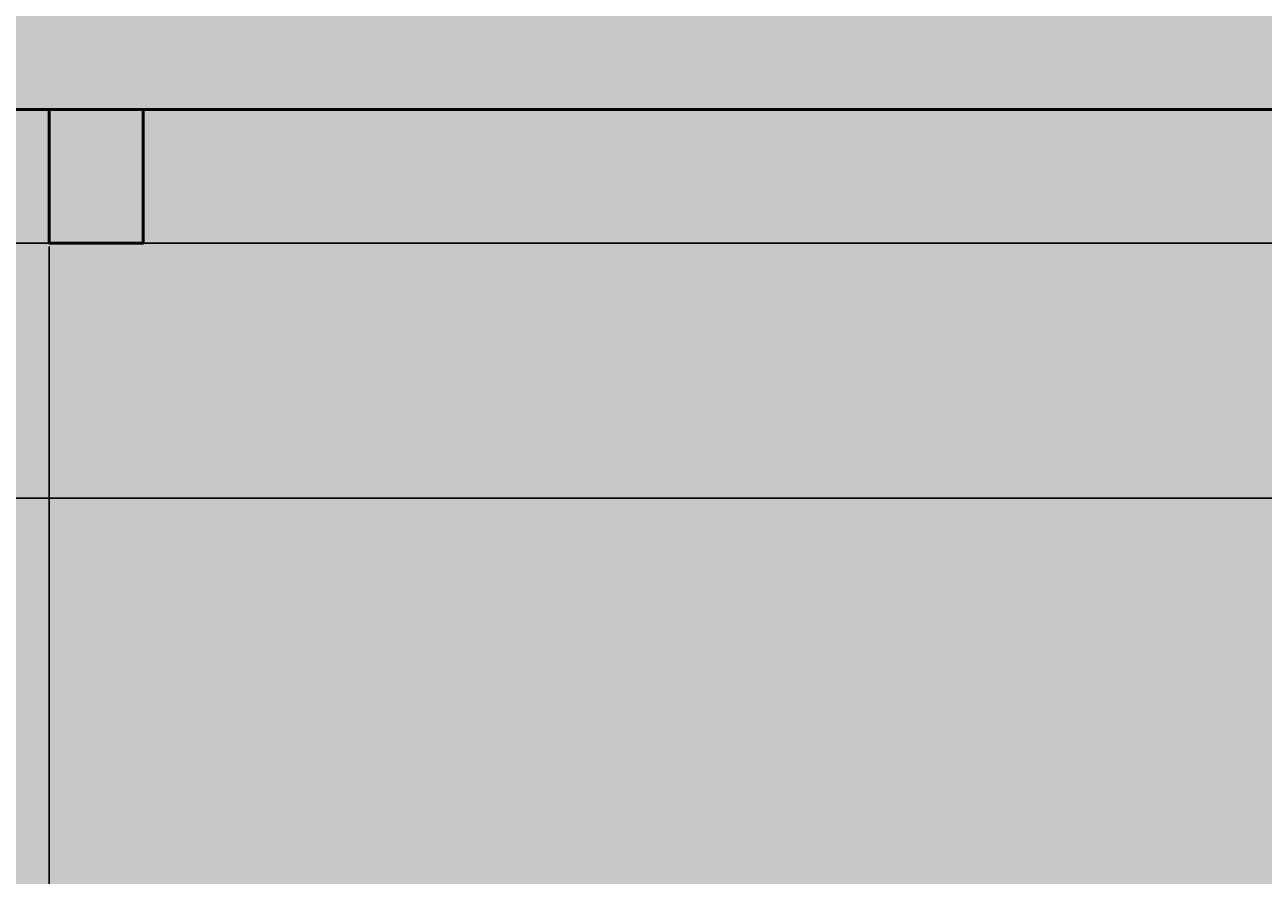
# Model space of a CAD drawing. Units: inches. Extents: x -12 to 334, y -10 to 186.
# Tile 37 of 77: x 129 to 152, y 49 to 65. Entities that reach past the tile are written whole.
import ezdxf

# ---------------------------------------------------------------- set-up
doc = ezdxf.new("R2010")
doc.units = ezdxf.units.IN
doc.header["$MEASUREMENT"] = 0
for name, color, linetype, lineweight in [('M-DIMS', 2, 'Continuous', 18), ('M-EQPM', 7, 'Continuous', 50), ('M-EQPM-PATT', 8, 'Continuous', 18)]:
    doc.layers.add(name, color=color, linetype=linetype, lineweight=lineweight)
doc.styles.get("Standard").update_dxf_attribs({"font": 'arial.ttf'})
doc.dimstyles.get("Standard").update_dxf_attribs({"dimtxt": 0.18, "dimasz": 0.18, "dimexe": 0.18, "dimexo": 0.0625, "dimgap": 0.09, "dimtad": 0, "dimtih": 1, "dimtoh": 1, "dimdec": 4, "dimzin": 0, "dimdsep": 46, "dimtxsty": 'Standard', "dimcen": 0.09, "dimadec": 0, "dimazin": 0, "dimtfac": 1, "dimtdec": 4, "dimtofl": 0, "dimtmove": 0, "dimatfit": 3, "dimfxl": 1, "dimtolj": 1, "dimtzin": 0, "dimarcsym": 0})

# ---------------------------------------------------------------- blocks, each defined once
blk = doc.blocks.new('*D1')
at = {"layer": 'Defpoints', "color": 0, "transparency": 16777216}
for p in [(281.426, 91.899), (3.376, 80.692), (281.426, 14.304)]:
    blk.add_point(p, dxfattribs=at)
at = {"layer": 'M-DIMS', "color": 0, "lineweight": -2, "transparency": 16777216}
for p, q in [((281.426, 91.836), (281.426, 14.124)), ((3.376, 80.629), (3.376, 14.124)), ((3.556, 14.304), (141.935, 14.304)), ((281.246, 14.304), (142.867, 14.304))]:
    blk.add_line(p, q, dxfattribs=at)
at = {"layer": 'M-DIMS', "color": 0, "transparency": 16777216}
for points in [[(3.556, 14.334), (3.556, 14.274), (3.376, 14.304)], [(281.246, 14.334), (281.246, 14.274), (281.426, 14.304)]]:
    blk.add_solid(points, dxfattribs=at)
at = {"layer": 'M-DIMS', "color": 0, "transparency": 16777216, "insert": (142.401, 14.304), "char_height": 0.18, "attachment_point": 5}
blk.add_mtext('\\A1;278.05', dxfattribs=at)
blk = doc.blocks.new('*D17')
at = {"layer": 'Defpoints', "color": 0, "transparency": 16777216}
for p in [(106.177, 102.896), (105.892, 56.321), (295.976, 56.321)]:
    blk.add_point(p, dxfattribs=at)
at = {"layer": 'M-DIMS', "color": 0, "lineweight": -2, "transparency": 16777216}
for p, q in [((106.24, 102.896), (296.156, 102.896)), ((295.976, 102.716), (295.976, 79.79)), ((295.976, 56.501), (295.976, 79.426)), ((105.954, 56.321), (296.156, 56.321))]:
    blk.add_line(p, q, dxfattribs=at)
at = {"layer": 'M-DIMS', "color": 0, "transparency": 16777216}
for points in [[(295.946, 102.716), (296.006, 102.716), (295.976, 102.896)], [(295.946, 56.501), (296.006, 56.501), (295.976, 56.321)]]:
    blk.add_solid(points, dxfattribs=at)
at = {"layer": 'M-DIMS', "color": 0, "transparency": 16777216, "insert": (295.976, 79.608), "char_height": 0.18, "attachment_point": 5}
blk.add_mtext('\\A1;46.575', dxfattribs=at)
blk = doc.blocks.new('*D30')
at = {"layer": 'Defpoints', "color": 0, "transparency": 16777216}
for p in [(75.924, 63.612), (129.093, 61.105), (129.093, 14.304)]:
    blk.add_point(p, dxfattribs=at)
at = {"layer": 'M-DIMS', "color": 0, "lineweight": -2, "transparency": 16777216}
for p, q in [((75.924, 63.549), (75.924, 14.124)), ((129.093, 61.042), (129.093, 14.124)), ((76.104, 14.304), (102.115, 14.304)), ((128.913, 14.304), (102.902, 14.304))]:
    blk.add_line(p, q, dxfattribs=at)
at = {"layer": 'M-DIMS', "color": 0, "transparency": 16777216}
for points in [[(76.104, 14.334), (76.104, 14.274), (75.924, 14.304)], [(128.913, 14.334), (128.913, 14.274), (129.093, 14.304)]]:
    blk.add_solid(points, dxfattribs=at)
at = {"layer": 'M-DIMS', "color": 0, "transparency": 16777216, "insert": (102.509, 14.304), "char_height": 0.18, "attachment_point": 5}
blk.add_mtext('\\A1;53.17', dxfattribs=at)
blk = doc.blocks.new('*D31')
at = {"layer": 'Defpoints', "color": 0, "transparency": 16777216}
for p in [(129.093, 61.105), (170.908, 61.105), (170.908, 14.304)]:
    blk.add_point(p, dxfattribs=at)
at = {"layer": 'M-DIMS', "color": 0, "lineweight": -2, "transparency": 16777216}
for p, q in [((129.093, 61.042), (129.093, 14.124)), ((170.908, 61.042), (170.908, 14.124)), ((129.273, 14.304), (149.532, 14.304)), ((170.728, 14.304), (150.468, 14.304))]:
    blk.add_line(p, q, dxfattribs=at)
at = {"layer": 'M-DIMS', "color": 0, "transparency": 16777216}
for points in [[(129.273, 14.334), (129.273, 14.274), (129.093, 14.304)], [(170.728, 14.334), (170.728, 14.274), (170.908, 14.304)]]:
    blk.add_solid(points, dxfattribs=at)
at = {"layer": 'M-DIMS', "color": 0, "transparency": 16777216, "insert": (150, 14.304), "char_height": 0.18, "attachment_point": 5}
blk.add_mtext('\\A1;41.815', dxfattribs=at)
blk = doc.blocks.new('*D35')
at = {"layer": 'Defpoints', "color": 0, "transparency": 16777216}
for p in [(216.428, 98.108), (-11.174, 61.105), (216.428, 61.105)]:
    blk.add_point(p, dxfattribs=at)
at = {"layer": 'M-DIMS', "color": 0, "lineweight": -2, "transparency": 16777216}
for p, q in [((216.365, 98.108), (-11.354, 98.108)), ((-11.174, 97.928), (-11.174, 79.788)), ((-11.174, 61.285), (-11.174, 79.424)), ((216.365, 61.105), (-11.354, 61.105))]:
    blk.add_line(p, q, dxfattribs=at)
at = {"layer": 'M-DIMS', "color": 0, "transparency": 16777216}
for points in [[(-11.204, 97.928), (-11.144, 97.928), (-11.174, 98.108)], [(-11.204, 61.285), (-11.144, 61.285), (-11.174, 61.105)]]:
    blk.add_solid(points, dxfattribs=at)
at = {"layer": 'M-DIMS', "color": 0, "transparency": 16777216, "insert": (-11.174, 79.606), "char_height": 0.18, "attachment_point": 5}
blk.add_mtext('\\A1;37', dxfattribs=at)
blk = doc.blocks.new('*D39')
at = {"layer": 'Defpoints', "color": 0, "transparency": 16777216}
for p in [(279.726, 80.692), (-11.174, 45.854), (269.381, 45.854)]:
    blk.add_point(p, dxfattribs=at)
at = {"layer": 'M-DIMS', "color": 0, "lineweight": -2, "transparency": 16777216}
for p, q in [((279.664, 80.692), (-11.354, 80.692)), ((-11.174, 80.512), (-11.174, 63.455)), ((-11.174, 46.034), (-11.174, 63.091)), ((269.318, 45.854), (-11.354, 45.854))]:
    blk.add_line(p, q, dxfattribs=at)
at = {"layer": 'M-DIMS', "color": 0, "transparency": 16777216}
for points in [[(-11.204, 80.512), (-11.144, 80.512), (-11.174, 80.692)], [(-11.204, 46.034), (-11.144, 46.034), (-11.174, 45.854)]]:
    blk.add_solid(points, dxfattribs=at)
at = {"layer": 'M-DIMS', "color": 0, "transparency": 16777216, "insert": (-11.174, 63.273), "char_height": 0.18, "attachment_point": 5}
blk.add_mtext('\\A1;34.84', dxfattribs=at)

msp = doc.modelspace()

# ---------------------------------------------------------------- hatches: boundary and pattern name
at = {"layer": 'M-EQPM-PATT'}
h = msp.add_hatch(color=256, dxfattribs=at)
h.set_gradient(color1=(205, 32, 39), color2=(205, 32, 39), tint=1)
h.paths.add_polyline_path([(64.5, 80.754), (64.5, 89.8963), (226.6083, 89.8963, -1), (226.6083, 69.6117), (64.5, 69.6117), (64.5, 78.754), (4.4744, 78.754, 0.384914), (23.5807, 61.4872), (37.1002, 61.4872), (37.1002, 33.6752), (53.1002, 33.6752), (53.1002, 61.4872), (64.5, 61.4872), (64.5, 63.6117), (226.6083, 63.6117, 1), (226.6083, 95.8963), (64.5, 95.8963), (64.5, 99.8958), (53.1002, 99.8958), (53.1002, 127.7078), (37.1002, 127.7078), (37.1002, 99.8958), (23.5807, 99.8958, 0.4132606), (4.3766, 80.754)])
h.paths.add_polyline_path([(64.5, 91.8963), (64.5, 93.8963), (226.6083, 93.8963, -1), (226.6083, 65.6117), (64.5, 65.6117), (64.5, 67.6117), (226.6083, 67.6117, 1), (226.6083, 91.8963)], flags=16)
h = msp.add_hatch(color=256, dxfattribs=at)
h.set_gradient(color1=(99, 100, 102), color2=(99, 100, 102), tint=1)
h.paths.add_polyline_path([(72.9244, 95.8963), (75.9244, 95.8963), (75.9244, 109.0583), (72.9244, 109.0583)])
h.paths.add_polyline_path([(72.9244, 50.4497), (75.9244, 50.4497), (75.9244, 63.6117), (72.9244, 63.6117)])
h.paths.add_polyline_path([(75.9244, 91.8963), (75.9244, 93.8963), (72.9244, 93.8963), (72.9244, 91.8963)])
h.paths.add_polyline_path([(75.9244, 65.6117), (75.9244, 67.6117), (72.9244, 67.6117), (72.9244, 65.6117)])
h.paths.add_polyline_path([(129.093, 69.6117), (130.8573, 69.6117), (130.8573, 89.8963), (129.093, 89.8963)])
h.paths.add_polyline_path([(129.093, 98.1081), (129.093, 95.8963), (130.8573, 95.8963), (130.8573, 98.1081)])
h.paths.add_polyline_path([(130.8573, 61.1045), (130.8573, 63.6117), (129.093, 63.6117), (129.093, 61.1045)])
h.paths.add_polyline_path([(170.9079, 69.6117), (172.6722, 69.6117), (172.6722, 89.8963), (170.9079, 89.8963)])
h.paths.add_polyline_path([(172.6722, 95.8963), (172.6722, 98.1081), (170.9079, 98.1081), (170.9079, 95.8963)])
h.paths.add_polyline_path([(170.9079, 61.1045), (172.6722, 61.1045), (172.6722, 63.6117), (170.9079, 63.6117)])
h.paths.add_polyline_path([(218.1922, 63.6117), (216.4278, 63.6117), (216.4278, 61.1045), (218.1922, 61.1045)])
h.paths.add_polyline_path([(216.4278, 69.6117), (218.1922, 69.6117), (218.1922, 89.8963), (216.4278, 89.8963)])
h.paths.add_polyline_path([(216.4278, 95.8963), (218.1922, 95.8963), (218.1922, 98.1081), (216.4278, 98.1081)])
h = msp.add_hatch(color=256, dxfattribs=at)
h.set_gradient(color1=(94, 103, 175), color2=(94, 103, 175), tint=1)
h.paths.add_polyline_path([(129.093, 89.8963), (86.8879, 89.8963), (86.8879, 69.6117), (129.093, 69.6117)], flags=17)
h.paths.add_polyline_path([(170.9079, 89.8963), (130.8573, 89.8963), (130.8573, 69.6117), (170.9079, 69.6117)], flags=17)
h.paths.add_polyline_path([(216.4278, 89.8963), (172.6722, 89.8963), (172.6722, 69.6117), (216.4278, 69.6117)], flags=17)
h.paths.add_polyline_path([(245.9354, 82.6969), (247.9354, 82.6969), (247.9354, 46.8541), (268.3808, 46.8541, 0.0998398), (279.7263, 80.6915), (251.9801, 80.6915, 0.4142136), (231.7758, 100.8958), (84.7229, 100.8958), (84.7229, 109.0583), (83.7229, 109.0583), (83.7229, 95.8963), (129.093, 95.8963), (129.093, 98.1081), (130.8573, 98.1081), (130.8573, 95.8963), (170.9079, 95.8963), (170.9079, 98.1081), (172.6722, 98.1081), (172.6722, 95.8963), (216.4278, 95.8963), (216.4278, 98.1081), (218.1922, 98.1081), (218.1922, 95.8963), (226.6083, 95.8963, -1), (226.6083, 63.6117), (218.1922, 63.6117), (218.1922, 61.1045), (216.4278, 61.1045), (216.4278, 63.6117), (172.6722, 63.6117), (172.6722, 61.1045), (170.9079, 61.1045), (170.9079, 63.6117), (130.8573, 63.6117), (130.8573, 61.1045), (129.093, 61.1045), (129.093, 63.6117), (87.8879, 63.6117), (87.8879, 56.3205), (105.8919, 56.3205), (105.8919, 28.8541), (115.8919, 28.8541), (115.8919, 46.8541), (222.5761, 46.8541), (222.5761, 30.8541), (232.5761, 30.8541), (232.5761, 46.8541), (245.9354, 46.8541)])
h.paths.add_polyline_path([(86.8879, 89.8963), (75.9244, 89.8963), (75.9244, 69.6117), (86.8879, 69.6117)])
h.paths.add_polyline_path([(83.7229, 109.0583), (75.9244, 109.0583), (75.9244, 95.8963), (83.7229, 95.8963)])
h.paths.add_polyline_path([(226.6083, 89.8963), (218.1922, 89.8963), (218.1922, 69.6117), (226.6083, 69.6117, 1)], flags=17)
h = msp.add_hatch(color=256, dxfattribs=at)
h.set_gradient(color1=(0, 0, 255), color2=(0, 0, 255), tint=1)
h.paths.add_polyline_path([(84.7229, 100.8958), (84.7229, 109.0583), (83.7229, 109.0583), (83.7229, 95.8963), (129.093, 95.8963), (129.093, 98.1081), (130.8573, 98.1081), (130.8573, 95.8963), (170.9079, 95.8963), (170.9079, 98.1081), (172.6722, 98.1081), (172.6722, 95.8963), (216.4278, 95.8963), (216.4278, 98.1081), (218.1922, 98.1081), (218.1922, 95.8963), (226.6083, 95.8963, -1), (226.6083, 63.6117), (218.1922, 63.6117), (218.1922, 61.1045), (216.4278, 61.1045), (216.4278, 63.6117), (172.6722, 63.6117), (172.6722, 61.1045), (170.9079, 61.1045), (170.9079, 63.6117), (130.8573, 63.6117), (130.8573, 61.1045), (129.093, 61.1045), (129.093, 63.6117), (87.8879, 63.6117), (87.8879, 56.3205), (105.8919, 56.3205), (105.8919, 28.8541), (115.8919, 28.8541), (115.8919, 46.8541), (222.5761, 46.8541), (222.5761, 30.8541), (232.5761, 30.8541), (232.5761, 46.8541), (245.9354, 46.8541), (245.9354, 82.6969), (247.9354, 82.6969), (247.9354, 46.8541), (268.3808, 46.8541, 0.0998398), (279.7263, 80.6915), (251.9801, 80.6915, 0.4142136), (231.7758, 100.8958)])

# ---------------------------------------------------------------- linework, layer by layer
at = {"layer": 'M-EQPM'}
msp.add_lwpolyline([(64.5, 63.6117), (226.6083, 63.6117, 1), (226.6083, 95.8963), (64.5, 95.8963)], format="xyb", dxfattribs=at)
msp.add_lwpolyline([(130.8573, 63.6117), (130.8573, 61.1045), (129.093, 61.1045), (129.093, 63.6117)], dxfattribs=at)

# ---------------------------------------------------------------- dimensions: what is measured, and where the dimension line sits
at = {"layer": 'M-DIMS'}
for base, p1, p2, override, picture, middle in [((295.9756, 56.3205), (106.1771, 102.8958), (105.8919, 56.3205), {"dimdec": 3, "dimlfac": 1, "dimrnd": 0, "dimzin": 0, "dimdsep": 46, "dimlunit": 2}, '*D17', (295.9756, 79.6082)), ((-11.1736, 61.1045), (216.4278, 98.1081), (216.4278, 61.1045), {"dimdec": 0, "dimlfac": 1, "dimrnd": 0, "dimzin": 0, "dimdsep": 46, "dimlunit": 2}, '*D35', (-11.1735, 79.6063)), ((-11.1736, 45.8541), (279.7263, 80.6915), (269.3808, 45.8541), {"dimdec": 2, "dimlfac": 1, "dimrnd": 0, "dimzin": 0, "dimdsep": 46, "dimlunit": 2}, '*D39', (-11.1735, 63.2728))]:
    dim = msp.add_linear_dim(base=base, p1=p1, p2=p2, angle=90, dimstyle='Standard', override=override, dxfattribs=at)
    dim.commit()
    dim.dimension.update_dxf_attribs({"geometry": picture, "text_midpoint": middle})
for base, p1, p2, override, picture, middle in [((281.4256, 14.3041), (3.3765, 80.6915), (281.4256, 91.8988), {"dimdec": 2, "dimlfac": 1, "dimrnd": 0, "dimzin": 0, "dimdsep": 46, "dimlunit": 2}, '*D1', (142.401, 14.3041)), ((129.093, 14.3041), (75.9244, 63.6117), (129.093, 61.1045), {"dimdec": 2, "dimlfac": 1, "dimrnd": 0, "dimzin": 0, "dimdsep": 46, "dimlunit": 2}, '*D30', (102.5087, 14.3041)), ((170.9079, 14.3041), (129.093, 61.1045), (170.9079, 61.1045), {"dimdec": 3, "dimlfac": 1, "dimrnd": 0, "dimzin": 0, "dimdsep": 46, "dimlunit": 2}, '*D31', (150.0004, 14.3041))]:
    dim = msp.add_linear_dim(base=base, p1=p1, p2=p2, dimstyle='Standard', override=override, dxfattribs=at)
    dim.commit()
    dim.dimension.update_dxf_attribs({"geometry": picture, "text_midpoint": middle})

doc.saveas('drawing.dxf')
